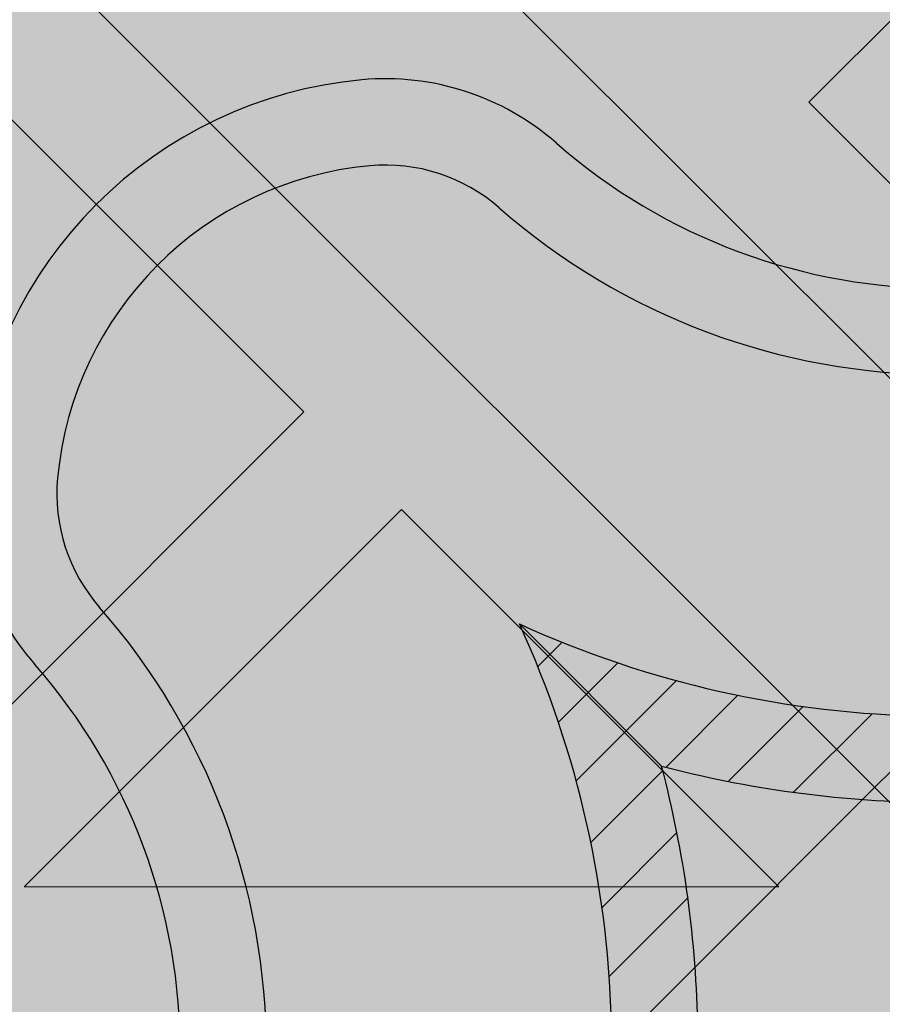
# Model space of a CAD drawing. Units: inches. Extents: x 844 to 2234, y 346 to 1084.
# Tile 17 of 93: x 1118.565 to 1120.159, y 703.242 to 705.06. Entities that reach past the tile are written whole.
import ezdxf

# ---------------------------------------------------------------- set-up
doc = ezdxf.new("R2010")
doc.units = ezdxf.units.IN
doc.header["$MEASUREMENT"] = 0
for name, color, linetype, lineweight in [('A-ANNO-DIMS', 2, 'Continuous', 18), ('furniture', 8, 'Continuous', 18), ('RA-AP-01$0$INT', 35, 'Continuous', 5)]:
    doc.layers.add(name, color=color, linetype=linetype, lineweight=lineweight)
doc.layers.add('RA-AP-01$0$FURN', color=3, linetype='Continuous')
doc.layers.add('RA-AP-01$0$WOOD', color=64, linetype='Continuous')
doc.styles.get("Standard").update_dxf_attribs({"font": 'arial.ttf'})
doc.dimstyles.get("Standard").update_dxf_attribs({"dimtxt": 6, "dimasz": 3, "dimexe": 0.18, "dimexo": 0.0625, "dimgap": 0.09, "dimtad": 0, "dimtih": 1, "dimtoh": 1, "dimdec": 1, "dimzin": 0, "dimdsep": 46, "dimlunit": 3, "dimtxsty": 'Standard', "dimblk": 'ARCHTICK', "dimcen": 0.09, "dimadec": 0, "dimazin": 0, "dimtfac": 1, "dimtdec": 1, "dimtofl": 0, "dimtmove": 0, "dimatfit": 3, "dimfxl": 1, "dimtolj": 1, "dimtzin": 0, "dimarcsym": 0})

# ---------------------------------------------------------------- blocks, each defined once
blk = doc.blocks.new('A$C18D01794')
at = {"layer": 'RA-AP-01$0$INT'}
h = blk.add_hatch(color=256, dxfattribs=at)
h.paths.add_polyline_path([(4.585917135068448, -7.856712009587804), (4.614201406330596, -7.856712009587056), (4.668846067270487, -7.802067348644738), (4.723490728212344, -7.856712009584164), (4.771774999457151, -7.856712009582887), (4.826419660396886, -7.80206734864072), (4.862780050090322, -7.838427738332541), (4.844495778842715, -7.856712009580965), (4.862780050090411, -7.856712009580482), (4.905206456960182, -7.814285602707865), (4.947632863832445, -7.856712009578238), (4.965917135079675, -7.856712009577755), (4.947632863831759, -7.838427738330656), (4.983993253523576, -7.802067348637219), (5.038637914464627, -7.856712009575829), (5.08692218571208, -7.856712009574554), (5.141566846649976, -7.802067348634224), (5.196211507589851, -7.856712009571666), (5.224495778822615, -7.856712009570916), (4.905206456953975, -7.537422687702283)])
h.paths.add_polyline_path([(4.895206456956031, -7.575706958950402), (4.895206456958921, -7.684996280828174), (4.840561796018589, -7.630351619890275)], flags=16)
h.paths.add_polyline_path([(4.915206456955638, -7.575706958949956), (4.969851117895509, -7.630351619887399), (4.915206456957609, -7.684996280827732)], flags=16)
h.paths.add_polyline_path([(4.826419660395175, -7.644493755514321), (4.881064321335613, -7.699138416452331), (4.771774999456703, -7.69913841645522)], flags=16)
h.paths.add_polyline_path([(4.983993253519558, -7.644493755510815), (5.038637914460456, -7.699138416449285), (4.929348592581548, -7.69913841645126)], flags=16)
h.paths.add_polyline_path([(4.881064321336025, -7.719138416452334), (4.826419660397532, -7.773783077393256), (4.771774999457062, -7.719138416455217)], flags=16)
h.paths.add_polyline_path([(4.929348592582019, -7.71913841645126), (5.038637914460982, -7.719138416449284), (4.983993253522945, -7.773783077389749)], flags=16)
h.paths.add_polyline_path([(4.895206456960191, -7.733280552075633), (4.895206456962115, -7.806001331460164), (4.876922185715016, -7.824285602708492), (4.840561796021581, -7.787925213016675)], flags=16)
h.paths.add_polyline_path([(4.915206456958487, -7.733280552075187), (4.969851117899527, -7.787925213013798), (4.933490728206909, -7.824285602708034), (4.9152064569598, -7.806001331461736)], flags=16)
h.paths.add_polyline_path([(4.757632863832376, -7.733280552079264), (4.812277524772842, -7.787925213017304), (4.757632863834348, -7.842569873958233)], flags=16)
h.paths.add_polyline_path([(4.737632863832376, -7.73328055207979), (4.737632863834348, -7.842569873958701), (4.682988202893906, -7.787925213020692)], flags=16)
h.paths.add_polyline_path([(5.05278005008503, -7.733280552072701), (5.052780050087917, -7.842569873951664), (4.998135389146995, -7.787925213013169)], flags=16)
h.paths.add_polyline_path([(5.072780050085024, -7.733280552072333), (5.127424711025931, -7.787925213010806), (5.072780050087916, -7.842569873951244)], flags=16)
h.paths.add_polyline_path([(4.935917135072783, -7.506712009583784), (5.255206456948811, -7.826001331459767), (5.255206456948932, -7.797717060211899), (5.200561796010279, -7.743072399273238), (5.255206456949403, -7.688427738334128), (5.25520645694961, -7.640143467086677), (5.200561796009787, -7.585498806146837), (5.236922185702417, -7.549138416454212), (5.255206456949919, -7.56742268770172), (5.255206456949998, -7.549138416454178), (5.212780050078687, -7.506712009583814), (5.25520645695036, -7.464285602712145), (5.255206456950438, -7.446001331464763), (5.236922185702424, -7.464285602712779), (5.200561796009796, -7.427925213020149), (5.255206456950753, -7.373280552079203), (5.25520645695096, -7.324996280834394), (5.200561796010322, -7.270351619893748), (5.255206456951428, -7.215706958952649), (5.255206456951547, -7.187422687705071)])
h.paths.add_polyline_path([(5.042988202883395, -7.42792521302065), (5.097632863823085, -7.373280552080975), (5.097632863822622, -7.482569873959883)], flags=16)
h.paths.add_polyline_path([(5.028846067259663, -7.442067348644384), (5.083490728198774, -7.496712009583504), (4.974201406321001, -7.496712009583035)], flags=16)
h.paths.add_polyline_path([(5.117632863823087, -7.37328055208089), (5.172277524762331, -7.42792521302015), (5.11763286382262, -7.482569873959851)], flags=16)
h.paths.add_polyline_path([(5.08349072819877, -7.516712009582191), (5.028846067259652, -7.571356670521302), (4.974201406320998, -7.516712009582638)], flags=16)
h.paths.add_polyline_path([(5.131774999446817, -7.35913841645716), (5.186419660386065, -7.413783077396415), (5.241064321325782, -7.359138416456712)], flags=17)
h.paths.add_polyline_path([(5.131774999446228, -7.496712009583703), (5.186419660386065, -7.442067348643883), (5.222780050079488, -7.478427738337313), (5.204495778832781, -7.496712009584014)], flags=16)
h.paths.add_polyline_path([(5.097632863822613, -7.530854145205813), (5.097632863823061, -7.640143467084723), (5.042988202883383, -7.585498806145032)], flags=16)
h.paths.add_polyline_path([(5.131774999446899, -7.339138416457162), (5.241064321325809, -7.339138416456712), (5.186419660386591, -7.284493755517479)], flags=17)
h.paths.add_polyline_path([(5.131774999446226, -7.516712009581999), (5.204495778830767, -7.516712009581702), (5.22278005007868, -7.534996280829206), (5.186419660386049, -7.571356670521828)], flags=16)
h.paths.add_polyline_path([(5.11763286382262, -7.530854145205852), (5.17227752476232, -7.585498806145562), (5.117632863823064, -7.64014346708481)], flags=16)
h.paths.add_polyline_path([(5.186419660386069, -7.599640941770585), (5.241064321325754, -7.654285602710281), (5.131774999446791, -7.654285602709814)], flags=16)
h.paths.add_polyline_path([(5.131774999446872, -7.674285602709813), (5.24106432132578, -7.674285602710282), (5.186419660386554, -7.728930263649504)], flags=16)
h.paths.add_polyline_path([(5.255206456951811, -7.126001331467467), (5.255206456951895, -7.106712009588038), (4.555206456956052, -7.106712009588038), (4.555206456956136, -7.12600133146746), (4.905206456953973, -7.476001331465289)])
h.paths.add_polyline_path([(4.983993253513404, -7.368930263651977), (4.92934859257295, -7.314285602713969), (5.03863791445186, -7.314285602711063)], flags=16)
h.paths.add_polyline_path([(4.969851117889988, -7.383072399276016), (4.915206456952556, -7.437717060215906), (4.915206456949648, -7.328427738338133)], flags=16)
h.paths.add_polyline_path([(4.929348592572535, -7.294285602713971), (4.983993253511019, -7.239640941773039), (5.038637914451496, -7.294285602711065)], flags=16)
h.paths.add_polyline_path([(5.052780050074912, -7.280143467087016), (4.998135389134438, -7.225498806148989), (5.052780050072919, -7.170854145208052)], flags=16)
h.paths.add_polyline_path([(5.07278005007491, -7.280143467086489), (5.072780050072918, -7.170854145207579), (5.127424711013374, -7.225498806145578)], flags=16)
h.paths.add_polyline_path([(4.89520645695295, -7.437717060216355), (4.840561796013067, -7.383072399278919), (4.895206456950961, -7.328427738338582)], flags=16)
h.paths.add_polyline_path([(4.915206456948365, -7.280143467090674), (4.915206456946434, -7.207422687704125), (4.933490728192729, -7.18913841645701), (4.969851117886972, -7.225498806149623)], flags=16)
h.paths.add_polyline_path([(4.881064321327021, -7.314285602715054), (4.82641966038902, -7.368930263655506), (4.771774999448108, -7.314285602717047)], flags=16)
h.paths.add_polyline_path([(4.895206456950073, -7.280143467091125), (4.840561796009022, -7.225498806152518), (4.876922185700835, -7.18913841645908), (4.895206456948749, -7.207422687706589)], flags=16)
h.paths.add_polyline_path([(4.983993253510392, -7.211356670525576), (4.947632863816944, -7.174996280833758), (4.965917135064043, -7.156712009585847), (5.038637914448995, -7.156712009584522)], flags=16)
h.paths.add_polyline_path([(4.881064321326543, -7.294285602715056), (4.771774999447578, -7.294285602717046), (4.826419660385607, -7.239640941776569)], flags=16)
h.paths.add_polyline_path([(4.905206456946447, -7.19913841645844), (4.862780050074785, -7.156712009587725), (4.947632863816685, -7.156712009586302)], flags=16)
h.paths.add_polyline_path([(5.14156684663679, -7.211356670521528), (5.086922185696452, -7.156712009583639), (5.196211507574223, -7.156712009581651)], flags=16)
h.paths.add_polyline_path([(4.8264196603837, -7.211356670529104), (4.771774999442643, -7.156712009590501), (4.8444957788276, -7.156712009588568), (4.862780050075511, -7.17499628083566)], flags=16)
h.paths.add_polyline_path([(4.812277524760289, -7.225498806153156), (4.757632863822258, -7.28014346709363), (4.757632863819352, -7.170854145214669)], flags=16)
h.paths.add_polyline_path([(4.73763286382226, -7.280143467093997), (4.682988202881349, -7.22549880615554), (4.737632863819352, -7.170854145215086)], flags=16)
h.paths.add_polyline_path([(4.723490728195188, -7.156712009591787), (4.668846067257299, -7.211356670532127), (4.614201406317417, -7.156712009594693)], flags=16)
h.paths.add_polyline_path([(4.597632863829262, -7.506712009583814), (4.555206456957951, -7.54913841645418), (4.555206456958029, -7.56742268770172), (4.573490728205535, -7.549138416454212), (4.609851117898167, -7.585498806146839), (4.555206456958338, -7.640143467086675), (4.555206456958546, -7.688427738334125), (4.60985111789767, -7.743072399273238), (4.555206456959015, -7.797717060211899), (4.555206456959138, -7.826001331459767), (4.874495778835167, -7.506712009583786), (4.5552064569564, -7.187422687705062), (4.555206456956523, -7.215706958952644), (4.609851117897629, -7.270351619893746), (4.555206456956988, -7.324996280834396), (4.555206456957198, -7.373280552079195), (4.609851117898153, -7.427925213020147), (4.573490728205528, -7.464285602712779), (4.555206456957507, -7.446001331464756), (4.555206456957585, -7.464285602712143)])
h.paths.add_polyline_path([(4.712780050085332, -7.482569873959882), (4.712780050084863, -7.373280552080972), (4.767424711024555, -7.42792521302065)], flags=16)
h.paths.add_polyline_path([(4.726922185709173, -7.496712009583504), (4.781566846648288, -7.442067348644384), (4.836211507586949, -7.496712009583033)], flags=16)
h.paths.add_polyline_path([(4.692780050085327, -7.482569873959851), (4.638135389145619, -7.427925213020149), (4.692780050084865, -7.373280552080892)], flags=16)
h.paths.add_polyline_path([(4.726922185709182, -7.516712009582191), (4.836211507586949, -7.51671200958264), (4.7815668466483, -7.571356670521304)], flags=16)
h.paths.add_polyline_path([(4.678637914461726, -7.496712009583706), (4.605917135075169, -7.496712009584014), (4.587632863828464, -7.478427738337311), (4.623993253521887, -7.442067348643881)], flags=16)
h.paths.add_polyline_path([(4.712780050085336, -7.530854145205816), (4.767424711024568, -7.585498806145034), (4.71278005008489, -7.640143467084724)], flags=16)
h.paths.add_polyline_path([(4.678637914461726, -7.516712009582001), (4.623993253521899, -7.571356670521829), (4.587632863829271, -7.534996280829206), (4.605917135077185, -7.5167120095817)], flags=16)
h.paths.add_polyline_path([(4.692780050085336, -7.530854145205848), (4.692780050084889, -7.64014346708481), (4.638135389145632, -7.585498806145562)], flags=16)
h.paths.add_polyline_path([(4.623993253521885, -7.413783077396415), (4.678637914461131, -7.359138416457161), (4.56934859258217, -7.359138416456712)], flags=17)
h.paths.add_polyline_path([(4.623993253521901, -7.599640941770568), (4.678637914461158, -7.654285602709814), (4.569348592582195, -7.654285602710281)], flags=16)
h.paths.add_polyline_path([(4.678637914461051, -7.339138416457162), (4.623993253521361, -7.284493755517479), (4.569348592582143, -7.339138416456712)], flags=17)
h.paths.add_polyline_path([(4.678637914461076, -7.674285602709813), (4.623993253521399, -7.728930263649504), (4.569348592582167, -7.674285602710281)], flags=16)
h = blk.add_hatch(color=256, dxfattribs=at)
h.paths.add_polyline_path([(4.905206456954232, -7.537422687702028), (4.874495778835232, -7.506712009583718), (4.555206456959138, -7.826001331459766), (4.555206456959269, -7.856712009588616), (4.585917135068449, -7.856712009587804)])
h.paths.add_polyline_path([(4.935917135072152, -7.506712009583152), (4.905206456953497, -7.537422687701806), (5.224495778822614, -7.856712009570917), (5.255206456948681, -7.856712009570104), (5.255206456948813, -7.826001331459768)])
h.paths.add_polyline_path([(5.255206456951549, -7.18742268770507), (5.255206456951813, -7.126001331467461), (4.905206456953563, -7.476001331465701), (4.935917135072559, -7.506712009584006)])
h.paths.add_polyline_path([(4.874495778835167, -7.506712009583785), (4.905206456953818, -7.476001331465132), (4.555206456956135, -7.126001331467458), (4.555206456956399, -7.187422687705064)])
h = blk.add_hatch(color=256, dxfattribs=at)
h.paths.add_polyline_path([(4.781566846647504, -7.442067348645805), (4.836211507586161, -7.496712009584463), (4.726922185708388, -7.496712009584918)])
h.paths.add_polyline_path([(4.836211507586161, -7.516712009584068), (4.781566846647504, -7.571356670522723), (4.726922185708388, -7.516712009583606)])
h.paths.add_polyline_path([(4.76742471102377, -7.585498806146453), (4.712780050084083, -7.640143467086137), (4.712780050084542, -7.530854145207227)])
h.paths.add_polyline_path([(4.692780050084544, -7.530854145207257), (4.692780050084084, -7.64014346708622), (4.638135389144834, -7.585498806146965)])
h.paths.add_polyline_path([(4.678637914460932, -7.516712009583407), (4.623993253521102, -7.571356670523233), (4.587632863827676, -7.53499628082981), (4.605917135074382, -7.516712009583104)])
h.paths.add_polyline_path([(4.573490728204743, -7.54913841645434), (4.60985111789737, -7.585498806146969), (4.555206456957541, -7.640143467086797), (4.555206456957237, -7.567422687701846)])
h.paths.add_polyline_path([(4.623993253521098, -7.599640941770699), (4.67863791446035, -7.654285602709951), (4.56934859258139, -7.654285602710407)])
h.paths.add_polyline_path([(4.678637914460275, -7.67428560270995), (4.623993253520583, -7.728930263649637), (4.56934859258136, -7.674285602710405)])
h.paths.add_polyline_path([(4.609851117896854, -7.743072399273369), (4.555206456958196, -7.797717060212026), (4.555206456957738, -7.688427738334254)])
h.paths.add_polyline_path([(4.597632863828475, -7.506712009583301), (4.555206456957283, -7.549138416454495), (4.555206456956805, -7.464285602712587)])
h.paths.add_polyline_path([(4.678637914460932, -7.496712009585113), (4.605917135076396, -7.496712009585417), (4.587632863828479, -7.478427738337913), (4.623993253521104, -7.442067348645284)])
h.paths.add_polyline_path([(4.692780050084091, -7.373280552082301), (4.692780050084548, -7.482569873961267), (4.638135389144834, -7.427925213021552)])
h.paths.add_polyline_path([(4.767424711023772, -7.427925213022072), (4.712780050084545, -7.48256987396129), (4.712780050084089, -7.373280552082384)])
h.paths.add_polyline_path([(4.67863791446036, -7.359138416457298), (4.623993253521105, -7.41378307739655), (4.569348592581399, -7.35913841645684)])
h.paths.add_polyline_path([(4.609851117897371, -7.427925213020278), (4.573490728204743, -7.464285602712907), (4.555206456957237, -7.446001331465401), (4.555206456957548, -7.373280552080448)])
h.paths.add_polyline_path([(4.623993253520596, -7.284493755517612), (4.67863791446028, -7.339138416457299), (4.569348592581367, -7.339138416456838)])
h.paths.add_polyline_path([(4.609851117896867, -7.270351619893878), (4.555206456957749, -7.324996280832994), (4.55520645695821, -7.21570695895522)])
h = blk.add_hatch(color=256, dxfattribs=at)
h.paths.add_polyline_path([(4.969851117891331, -7.630351619889621), (4.915206456952669, -7.575706958950966), (4.915206456952222, -7.684996280828739)])
h.paths.add_polyline_path([(4.895206456953064, -7.575706958950968), (4.840561796014413, -7.630351619889628), (4.895206456953533, -7.684996280828741)])
h.paths.add_polyline_path([(4.826419660390684, -7.644493755513362), (4.771774999451003, -7.699138416453052), (4.881064321329913, -7.699138416452587)])
h.paths.add_polyline_path([(4.881064321329884, -7.719138416452585), (4.771774999450921, -7.719138416453052), (4.82641966039018, -7.773783077392298)])
h.paths.add_polyline_path([(4.895206456953734, -7.733280552076196), (4.840561796013912, -7.787925213016031), (4.876922185707337, -7.824285602709455), (4.895206456954043, -7.806001331462747)])
h.paths.add_polyline_path([(4.862780050082808, -7.838427738332388), (4.826419660390178, -7.802067348639763), (4.771774999450351, -7.856712009579595), (4.844495778835303, -7.856712009579895)])
h.paths.add_polyline_path([(4.812277524766446, -7.787925213016036), (4.757632863827191, -7.733280552076788), (4.757632863826741, -7.842569873955747)])
h.paths.add_polyline_path([(4.737632863827191, -7.733280552076863), (4.682988202887508, -7.787925213016558), (4.737632863826743, -7.842569873955778)])
h.paths.add_polyline_path([(4.668846067263777, -7.802067348640287), (4.614201406325123, -7.856712009578949), (4.723490728202894, -7.856712009579402)])
h.paths.add_polyline_path([(4.905206456953846, -7.814285602708654), (4.862780050082654, -7.856712009579847), (4.947632863824561, -7.85671200958032)])
h.paths.add_polyline_path([(4.915206456952028, -7.733280552076195), (4.91520645695173, -7.806001331460731), (4.933490728199234, -7.824285602708648), (4.96985111789186, -7.787925213016022)])
h.paths.add_polyline_path([(5.038637914454841, -7.719138416453029), (4.929348592575874, -7.71913841645258), (4.983993253515593, -7.773783077392289)])
h.paths.add_polyline_path([(4.983993253515065, -7.644493755513352), (4.929348592575849, -7.699138416452582), (5.038637914454755, -7.699138416453031)])
h.paths.add_polyline_path([(5.052780050079843, -7.73328055207676), (4.998135389140595, -7.787925213016018), (5.052780050080309, -7.842569873955721)])
h.paths.add_polyline_path([(4.983993253516868, -7.802067348639752), (4.947632863824241, -7.838427738332383), (4.965917135071747, -7.856712009579888), (5.038637914456701, -7.856712009579572)])
h.paths.add_polyline_path([(5.127424711019533, -7.787925213016519), (5.072780050079843, -7.733280552076838), (5.07278005008031, -7.842569873955751)])
h.paths.add_polyline_path([(5.141566846643269, -7.802067348640248), (5.086922185704154, -7.85671200957937), (5.196211507581929, -7.856712009578901)])
for p, q in [((4.874495778835167, -7.506712009583786), (4.555206456959136, -7.826001331459769)), ((4.905206456953975, -7.537422687702283), (4.585917135071132, -7.856712009585121)), ((4.569348592582168, -7.674285602710281), (4.623993253521399, -7.728930263649504)), ((4.678637914461078, -7.674285602709813), (4.569348592582168, -7.674285602710281)), ((4.6239932535214, -7.728930263649502), (4.678637914461078, -7.674285602709813)), ((4.555206456958551, -7.68842773833413), (4.60985111789767, -7.743072399273238)), ((4.682988202893908, -7.78792521302069), (4.737632863832376, -7.733280552079792)), ((4.555206456959017, -7.797717060211899), (4.60985111789767, -7.743072399273238)), ((4.737632863834348, -7.842569873958701), (4.682988202893906, -7.787925213020692))]:
    blk.add_line(p, q, dxfattribs=at)
blk = doc.blocks.new('A$C32926AE1')
at = {"layer": 'RA-AP-01$0$WOOD'}
h = blk.add_hatch(color=256, dxfattribs=at)
h.dxf.hatch_style = 1
h.paths.add_polyline_path([(5.157430609644524, 4.573483066760929, -0.1009492694046607), (5.155401577623758, 4.593365984175333, -0.1842662638101597), (5.172249623284174, 4.638795604568598, 0.2056608120311276), (5.179560981299304, 4.661316324430096, 0.3614336704623542), (5.134352340494423, 4.706524965234944, 0.2056608120311297), (5.111831620632933, 4.699213607219793, -0.1842662638101113), (5.066402000239693, 4.682365561559342, -0.1055311479399994), (5.045656153913092, 4.68467289944697, 0.1567636581983829), (4.763886414745334, 4.684672899446966, -0.1055311479399895), (4.743140568418733, 4.68236556155934, -0.1842662638100833), (4.6977109480255, 4.69921360721979, 0.2056608120302612), (4.675190228164109, 4.706524965234949, 0.3614336704708441), (4.629981587358889, 4.66131632442871, 0.2056608120245944), (4.637292945374126, 4.638795604567974, -0.1842662638101024), (4.654140991034615, 4.59336598417475, -0.1009492694055169), (4.652111959013835, 4.573483066760181, 0.021410119221476), (4.629748025606143, 4.156712009541676, 0.0214101192214795), (4.652111959013809, 3.739940952323101, -0.1009492694059586), (4.654140991034615, 3.720058034908448, -0.1842662638100975), (4.637292945374126, 3.674628414515226, 0.2056608120245705), (4.629981587358889, 3.652107694654492, 0.3614336704708879), (4.675190228164113, 3.606899053848249, 0.2056608120302384), (4.697710948025501, 3.614210411863408, -0.1842662638100995), (4.743140568418738, 3.63105845752386, -0.1055311479402541), (4.763886414745388, 3.628751119636215, 0.1567636581983776), (5.045656153913137, 3.628751119636244, -0.1055311479397538), (5.066402000239692, 3.631058457523857, -0.1842662638101067), (5.111831620632931, 3.614210411863407, 0.2056608120310924), (5.134352340494417, 3.606899053848256, 0.3614336704624001), (5.179560981299307, 3.652107694653103, 0.2056608120311314), (5.172249623284175, 3.6746284145146, -0.1842662638101402), (5.155401577623758, 3.72005803490786, -0.1009492694051366), (5.15743060964455, 3.739940952322354, 0.0214101192215073), (5.179794543052287, 4.156712009541468, 0.0214101192215252)])
h.paths.add_polyline_path([(4.639748609479751, 4.156712009541513, 0.0213537860821624), (4.661970494867118, 3.741887061152232, -0.094075836301374), (4.664143710413708, 3.7196126951003, -0.1824818158568985), (4.644813765429836, 3.668037719127816, 0.2056608120245319), (4.639939526753007, 3.653023905887301, 0.3614336704710246), (4.676106439397173, 3.616856993242342, 0.2056608120302234), (4.691120252638095, 3.621731231919122, -0.1824818158602558), (4.742695228611606, 3.641061176902986, -0.1029891339458722), (4.766991894714349, 3.638256818950944, 0.156709409989566), (5.042550673941472, 3.638256818950105, -0.102989133958497), (5.066847340047078, 3.641061176902949, -0.1824818158594995), (5.118422316020358, 3.621731231919103, 0.2056608120311416), (5.133436129261316, 3.616856993242346, 0.3614336704621468), (5.169603041905217, 3.653023905886178, 0.2056608120310986), (5.164728803228477, 3.668037719127177, -0.1824818158565612), (5.145398858244737, 3.719612695099578, -0.0940758363009313), (5.147572073791232, 3.741887061151398, 0.0213537860822023), (5.169793959178681, 4.156712009541451, 0.0213537860822226), (5.147572073791203, 4.571536957931898, -0.0940758363005034), (5.145398858244737, 4.59381132398362, -0.1824818158565587), (5.164728803228476, 4.645386299956021, 0.2056608120311045), (5.169603041905216, 4.66040011319702, 0.3614336704621845), (5.133436129261313, 4.696567025840856, 0.2056608120310773), (5.118422316020359, 4.691692787164098, -0.182481815859508), (5.066847340047078, 4.67236284218025, -0.1029891339584606), (5.04255067394148, 4.675167200133092, 0.156709409989566), (4.766991894714357, 4.675167200132257, -0.1029891339458842), (4.742695228611611, 4.672362842180213, -0.1824818158602725), (4.691120252638095, 4.691692787164077, 0.2056608120302152), (4.676106439397174, 4.696567025840858, 0.3614336704710363), (4.639939526753005, 4.660400113195899, 0.2056608120245495), (4.644813765429837, 4.645386299955384, -0.1824818158568934), (4.664143710413708, 4.593811323982902, -0.0940758363009187), (4.661970494867149, 4.571536957931074, 0.021353786082177)], flags=16)
h.paths.add_polyline_path([(5.129794543052235, 4.432167055276933, -0.0141661062790638), (5.130152669293814, 4.156927903047693, -0.0141661062790647), (5.129794543052234, 3.881688750818433, -0.0785247771143638), (5.10979738006795, 3.755143611847103, 0.0945969212073497), (5.105408519571111, 3.717898134952927, 0.1043170707844957), (5.116074640131521, 3.670385395016088, 0.1043170707864965), (5.068561900193738, 3.681051515576561, 0.09459692119553), (5.031316423304057, 3.676662655080835, -0.1580239521427272), (4.778226145355827, 3.676662655080367, 0.0945969211986668), (4.740980668464973, 3.681051515576592, 0.1043170707882822), (4.693467928526415, 3.670385395015844, 0.1043170707867916), (4.704134049087309, 3.717898134953662, 0.0945969211972894), (4.69974518859162, 3.755143611844042, -0.0785247771163196), (4.679748025606343, 3.881688750818406, -0.0141661062790663), (4.679389899364763, 4.156927903047693, -0.0141661062790672), (4.679748025606343, 4.432167055276998, -0.0785247771163064), (4.699745188591625, 4.55871219425134, 0.094596921197333), (4.704134049087308, 4.595957671141738, 0.1043170707867205), (4.693467928526416, 4.643470411079523, 0.1043170707882628), (4.740980668464965, 4.632804290518776, 0.0945969211988114), (4.778226145355874, 4.637193151015016, -0.158023952142669), (5.031316423304015, 4.637193151014546, 0.0945969211956361), (5.068561900193736, 4.632804290518806, 0.1043170707864979), (5.11607464013152, 4.643470411079278, 0.1043170707844617), (5.105408519571112, 4.595957671142455, 0.0945969212074597), (5.109797380067959, 4.558712194248236, -0.0785247771143467)], flags=0)
h.paths.add_polyline_path([(5.119794532311105, 4.432259799204851, -0.0142000800617244), (5.120156169157484, 4.156927903047701, -0.0142000800617277), (5.119794532311105, 3.881596006890482, -0.0784894509520253), (5.100273383573699, 3.758192358677797, 0.0940138827242913), (5.095413455884425, 3.717477693979438, 0.0606271852308753), (5.099615656341024, 3.686844378806616, 0.0606271852322524), (5.068982341167493, 3.691046579263239, 0.0940138827010453), (5.028267676478798, 3.686186651576848, -0.1580706864508061), (4.781274892180912, 3.686186651576435, 0.0940138827026903), (4.740560227491556, 3.691046579263279, 0.0606271852339895), (4.709926912317155, 3.686844378806508, 0.0606271852329405), (4.714129112773991, 3.717477693980356, 0.094013882701304), (4.709269185087677, 3.758192358669163, -0.0784894509577193), (4.689748036347473, 3.881596006890469, -0.014200080061729), (4.689386399501094, 4.156927903047709, -0.0142000800617217), (4.689748036347473, 4.432259799204808, -0.078489450957724), (4.709269185087651, 4.555663447426125, 0.0940138827014585), (4.714129112773992, 4.596378112114996, 0.0606271852329731), (4.709926912317154, 4.62701142728886, 0.0606271852340196), (4.74056022749157, 4.622809226832087, 0.0940138827024997), (4.781274892180847, 4.627669154518912, -0.1580706864508359), (5.028267676478777, 4.627669154518526, 0.0940138827010946), (5.068982341167492, 4.622809226832129, 0.060627185232254), (5.099615656341024, 4.627011427288751, 0.0606271852308727), (5.095413455884425, 4.59637811211593, 0.0940138827241088), (5.100273383573675, 4.555663447417647, -0.0784894509520978)], flags=0)
h.paths.add_polyline_path([(5.06978912287499, 4.430218106756144, -0.014241683694547), (5.070173729147532, 4.156927903047672, -0.0142416836945458), (5.06978912287499, 3.883637699339223, -0.0800609523125196), (5.052662118612511, 3.773463122773442, 0.0526421978001116), (5.04590916754064, 3.740550867606997, 0.0526421977992423), (5.012996912374707, 3.73379791653534, -0.1583028414718258), (4.796545656286308, 3.73379791653451, 0.0526421978034211), (4.763633401117837, 3.740550867607021, 0.0526421978018622), (4.756880450045755, 3.773463122774558, -0.0800609523117106), (4.739753445783639, 3.883637699339268, -0.0142416836945435), (4.739368839511098, 4.156927903047671, -0.0142416836945477), (4.739753445783639, 4.430218106756155, -0.0800609523116345), (4.75688045004574, 4.540392683320762, 0.052642197801941), (4.763633401117837, 4.573304938488346, 0.0526421978035071), (4.796545656286361, 4.580057889560873, -0.1583028414717561), (5.012996912374669, 4.580057889560039, 0.0526421977993048), (5.04590916754064, 4.57330493848837, 0.0526421978002057), (5.052662118612529, 4.540392683321868, -0.080060952312477)], flags=0)
h.paths.add_polyline_path([(5.049789715110557, 4.43038092723357, -0.0143097550741839), (5.05018085590259, 4.156927903047715, -0.0143097550741854), (5.049789715110558, 3.883474878861827, -0.0800685599149176), (5.03362098255317, 3.779581877367999, 0.0306258898956367), (5.028241146483733, 3.758218888663947, 0.0306258898977031), (5.006878157778253, 3.75283905259408, -0.1583983521624096), (4.802664410878162, 3.752839052594731, 0.0306258898946014), (4.781301422174808, 3.758218888663924, 0.0306258898967912), (4.775921586105202, 3.779581877368794, -0.080068559914251), (4.759752853548071, 3.883474878861786, -0.0143097550741854), (4.759361712756037, 4.156927903047671, -0.0143097550741854), (4.759752853548071, 4.430380927233557, -0.0800685599142479), (4.775921586105193, 4.534273928726546, 0.0306258898968306), (4.781301422174808, 4.555636917431444, 0.0306258898945754), (4.802664410878143, 4.561016753500631, -0.1583983521624168), (5.006878157778244, 4.561016753501291, 0.0306258898977177), (5.028241146483733, 4.555636917431421, 0.0306258898958182), (5.03362098255321, 4.534273928727244, -0.080068559914796)], flags=0)
h.paths.add_polyline_path([(4.999766070382627, 4.428171244713864, -0.0143443147609634), (5.000198441819402, 4.156927903047689, -0.0143443147609612), (4.999766070382627, 3.885684561381556, -0.0784641635803329), (4.987356730658798, 3.799103304488872, -0.1506053783831347), (4.822185837999821, 3.79910330448882, -0.0784641635803318), (4.809776498276007, 3.885684561381509, -0.014344314760963), (4.809344126839227, 4.156927903047677, -0.0143443147609645), (4.809776498276007, 4.428171244713873, -0.0784641635803192), (4.822185837999822, 4.514752501606549, -0.1506053783831338), (4.987356730658798, 4.514752501606494, -0.078464163580285)], flags=0)
h.paths.add_polyline_path([(4.979755254238824, 4.42764379880488, -0.0143772539198268), (4.980205517789977, 4.156927903047693, -0.0143772539198275), (4.979755254238824, 3.886212007290489, -0.0689242507424422), (4.971183264704897, 3.815276770442801, -0.1296645318904179), (4.838359303953726, 3.815276770442746, -0.0689242507424186), (4.829787314419809, 3.886212007290419, -0.0143772539198292), (4.829337050868653, 4.156927903047653, -0.0143772539198325), (4.829787314419809, 4.427643798804946, -0.0689242507424211), (4.838359303953725, 4.498579035652621, -0.1296645318904187), (4.971183264704897, 4.498579035652565, -0.0689242507424401)], flags=0)
h = blk.add_hatch(color=256, dxfattribs=at)
h.dxf.hatch_style = 1
h.paths.add_polyline_path([(5.145398858244737, 4.59381132398362, -0.1824818158565616), (5.164728803228476, 4.645386299956021, 0.2056608120311045), (5.169603041905216, 4.66040011319702, 0.3614336704621845), (5.133436129261313, 4.696567025840856, 0.2056608120310773), (5.118422316020359, 4.691692787164098, -0.182481815859508), (5.066847340047078, 4.67236284218025, -0.1029891339584606), (5.04255067394148, 4.675167200133092, 0.156709409989566), (4.766991894714357, 4.675167200132257, -0.1029891339458842), (4.742695228611611, 4.672362842180213, -0.1824818158602725), (4.691120252638095, 4.691692787164077, 0.2056608120302152), (4.676106439397174, 4.696567025840858, 0.3614336704710363), (4.639939526753005, 4.660400113195899, 0.2056608120245495), (4.644813765429837, 4.645386299955384, -0.1824818158568934), (4.664143710413708, 4.593811323982902, -0.0940758363009187), (4.661970494867149, 4.571536957931074, 0.0213537860821772), (4.639748609479751, 4.156712009541507, 0.0213537860821625), (4.661970494867119, 3.741887061152226, -0.0940758363013071), (4.664143710413708, 3.719612695100309, -0.1824818158569294), (4.644813765429836, 3.668037719127816, 0.2056608120245319), (4.639939526753007, 3.653023905887301, 0.3614336704710246), (4.676106439397173, 3.616856993242342, 0.2056608120302234), (4.691120252638095, 3.621731231919122, -0.1824818158602558), (4.742695228611606, 3.641061176902986, -0.1029891339458722), (4.766991894714349, 3.638256818950944, 0.156709409989566), (5.042550673941472, 3.638256818950105, -0.102989133958497), (5.066847340047078, 3.641061176902949, -0.1824818158594995), (5.118422316020358, 3.621731231919103, 0.2056608120311416), (5.133436129261316, 3.616856993242346, 0.3614336704621468), (5.169603041905217, 3.653023905886178, 0.2056608120310986), (5.164728803228477, 3.668037719127177, -0.1824818158565612), (5.145398858244737, 3.719612695099578, -0.0940758363009313), (5.147572073791232, 3.741887061151398, 0.0213537860822023), (5.169793959178681, 4.156712009541451, 0.0213537860822226), (5.147572073791203, 4.571536957931898, -0.0940758363004996)])
h.paths.add_polyline_path([(5.109797380067958, 4.55871219424824, -0.0785247771143472), (5.129794543052234, 4.432167055276936, -0.0141661062790644), (5.130152669293814, 4.156927903047685, -0.014166106279066), (5.129794543052234, 3.881688750818401, -0.0785247771143517), (5.109797380067946, 3.755143611847092, 0.0945969212073132), (5.105408519571111, 3.717898134952929, 0.1043170707844995), (5.116074640131521, 3.670385395016088, 0.1043170707864965), (5.068561900193738, 3.681051515576561, 0.09459692119553), (5.031316423304057, 3.676662655080835, -0.1580239521427272), (4.778226145355827, 3.676662655080367, 0.0945969211986668), (4.740980668464973, 3.681051515576592, 0.1043170707882822), (4.693467928526415, 3.670385395015844, 0.1043170707867916), (4.704134049087309, 3.717898134953662, 0.0945969211972894), (4.69974518859162, 3.755143611844042, -0.0785247771163196), (4.679748025606343, 3.881688750818406, -0.0141661062790663), (4.679389899364763, 4.156927903047693, -0.0141661062790672), (4.679748025606343, 4.432167055276998, -0.0785247771163064), (4.699745188591625, 4.55871219425134, 0.094596921197333), (4.704134049087308, 4.595957671141738, 0.1043170707867205), (4.693467928526416, 4.643470411079523, 0.1043170707882628), (4.740980668464965, 4.632804290518776, 0.0945969211988114), (4.778226145355874, 4.637193151015016, -0.158023952142669), (5.031316423304015, 4.637193151014546, 0.0945969211956361), (5.068561900193736, 4.632804290518806, 0.1043170707864979), (5.11607464013152, 4.643470411079278, 0.1043170707844617), (5.105408519571112, 4.595957671142455, 0.0945969212074504)], flags=16)
h.paths.add_polyline_path([(5.100273383573655, 4.55566344741771, -0.0784894509521388), (5.119794532311105, 4.432259799204852, -0.0142000800617252), (5.120156169157484, 4.156927903047686, -0.014200080061726), (5.119794532311105, 3.881596006890502, -0.0784894509520446), (5.100273383573696, 3.758192358677786, 0.0940138827242721), (5.095413455884425, 3.717477693979436, 0.0606271852308692), (5.099615656341024, 3.686844378806616, 0.0606271852322522), (5.068982341167493, 3.691046579263239, 0.0940138827010453), (5.028267676478798, 3.686186651576848, -0.1580706864508061), (4.781274892180912, 3.686186651576435, 0.0940138827026903), (4.740560227491556, 3.691046579263279, 0.0606271852339895), (4.709926912317155, 3.686844378806508, 0.0606271852329405), (4.714129112773991, 3.717477693980356, 0.094013882701304), (4.709269185087677, 3.758192358669163, -0.0784894509577193), (4.689748036347473, 3.881596006890469, -0.014200080061729), (4.689386399501094, 4.156927903047709, -0.0142000800617217), (4.689748036347473, 4.432259799204808, -0.078489450957724), (4.709269185087651, 4.555663447426125, 0.0940138827014585), (4.714129112773992, 4.596378112114996, 0.0606271852329731), (4.709926912317154, 4.62701142728886, 0.0606271852340196), (4.74056022749157, 4.622809226832087, 0.0940138827024997), (4.781274892180847, 4.627669154518912, -0.1580706864508359), (5.028267676478777, 4.627669154518526, 0.0940138827010946), (5.068982341167492, 4.622809226832129, 0.060627185232254), (5.099615656341024, 4.627011427288751, 0.0606271852308727), (5.095413455884425, 4.59637811211593, 0.094013882723957)], flags=0)
h.paths.add_polyline_path([(5.04590916754064, 4.57330493848837, 0.0526421978002057), (5.052662118612529, 4.540392683321868, -0.0800609523124783), (5.06978912287499, 4.430218106756142, -0.0142416836945469), (5.070173729147532, 4.156927903047672, -0.0142416836945458), (5.06978912287499, 3.883637699339223, -0.0800609523125196), (5.052662118612511, 3.773463122773442, 0.0526421978001116), (5.04590916754064, 3.740550867606997, 0.0526421977992423), (5.012996912374707, 3.73379791653534, -0.1583028414718258), (4.796545656286308, 3.73379791653451, 0.0526421978034211), (4.763633401117837, 3.740550867607021, 0.0526421978018622), (4.756880450045755, 3.773463122774558, -0.0800609523117106), (4.739753445783639, 3.883637699339268, -0.0142416836945435), (4.739368839511098, 4.156927903047671, -0.0142416836945477), (4.739753445783639, 4.430218106756155, -0.0800609523116345), (4.75688045004574, 4.540392683320762, 0.052642197801941), (4.763633401117837, 4.573304938488346, 0.0526421978035071), (4.796545656286361, 4.580057889560873, -0.1583028414717561), (5.012996912374669, 4.580057889560039, 0.0526421977993048)], flags=0)
h.paths.add_polyline_path([(5.028241146483733, 4.555636917431422, 0.0306258898956949), (5.033620982553182, 4.534273928727329, -0.0800685599148649), (5.049789715110557, 4.430380927233569, -0.0143097550741839), (5.05018085590259, 4.156927903047715, -0.0143097550741854), (5.049789715110558, 3.883474878861827, -0.0800685599149176), (5.03362098255317, 3.779581877367999, 0.0306258898956367), (5.028241146483733, 3.758218888663947, 0.0306258898977031), (5.006878157778253, 3.75283905259408, -0.1583983521624096), (4.802664410878162, 3.752839052594731, 0.0306258898946014), (4.781301422174808, 3.758218888663924, 0.0306258898967912), (4.775921586105202, 3.779581877368794, -0.080068559914251), (4.759752853548071, 3.883474878861786, -0.0143097550741854), (4.759361712756037, 4.156927903047671, -0.0143097550741854), (4.759752853548071, 4.430380927233557, -0.0800685599142479), (4.775921586105193, 4.534273928726546, 0.0306258898968306), (4.781301422174808, 4.555636917431444, 0.0306258898945754), (4.802664410878143, 4.561016753500631, -0.1583983521624168), (5.006878157778244, 4.561016753501291, 0.0306258898977174)], flags=0)
h.paths.add_polyline_path([(4.987356730658798, 4.514752501606494, -0.0784641635803018), (4.999766070382627, 4.428171244713845, -0.0143443147609637), (5.000198441819402, 4.156927903047665, -0.0143443147609622), (4.999766070382628, 3.885684561381514, -0.0784641635802952), (4.987356730658797, 3.799103304488872, -0.1506053783831338), (4.822185837999821, 3.799103304488819, -0.0784641635803342), (4.809776498276007, 3.885684561381512, -0.0143443147609628), (4.809344126839227, 4.156927903047676, -0.0143443147609646), (4.809776498276007, 4.428171244713873, -0.0784641635803192), (4.822185837999822, 4.514752501606549, -0.1506053783831338)], flags=0)
h.paths.add_polyline_path([(4.971183264704897, 4.498579035652566, -0.0689242507424384), (4.979755254238824, 4.427643798804883, -0.0143772539198276), (4.980205517789977, 4.15692790304768, -0.0143772539198258), (4.979755254238823, 3.88621200729051, -0.0689242507424628), (4.971183264704897, 3.815276770442801, -0.129664531890417), (4.838359303953726, 3.815276770442746, -0.0689242507424186), (4.829787314419809, 3.886212007290419, -0.0143772539198292), (4.829337050868653, 4.156927903047653, -0.0143772539198325), (4.829787314419809, 4.427643798804946, -0.0689242507424211), (4.838359303953725, 4.498579035652621, -0.1296645318904187)], flags=0)
h = blk.add_hatch(dxfattribs=at)
h.set_pattern_fill('ANSI31', color=256, scale=0.05, style=0)
h.set_pattern_definition([(45, (0, 0), (-0.0044194173824159, 0.0044194173824159), [])])
h.paths.add_polyline_path([(5.130152669293814, 4.156927903047704, 0.0141661062790657), (5.129794543052234, 4.432167055276982, 0.0777827904001433), (5.110168979996553, 4.557559993161921, -0.0976515123401879), (5.105408519571111, 4.595957671142454, -0.1043170707844687), (5.116074640131522, 4.64347041107928), (5.099615656341024, 4.627011427288751, 0.0606271852308727), (5.095413455884425, 4.59637811211593, 0.0940138827241088), (5.100273383573675, 4.555663447417647, -0.0784894509520972), (5.119794532311105, 4.432259799204852, -0.0142000800617252), (5.120156169157484, 4.156927903047686, -0.014200080061726), (5.119794532311105, 3.881596006890502, -0.0784894509520446), (5.100273383573696, 3.758192358677786, 0.0940138827242721), (5.095413455884425, 3.717477693979436, 0.0606271852308692), (5.099615656341024, 3.686844378806616), (5.116074640131519, 3.67038539501609, -0.1043170707844594), (5.105408519571112, 3.717898134952912, -0.0976515123401594), (5.11016897999655, 3.756295812933435, 0.0777827904001654), (5.129794543052234, 3.881688750818409, 0.0141661062790665)])
h.paths.add_polyline_path([(5.030164222210597, 3.676291055149937, -0.0976515123472002), (5.068561900193739, 3.681051515576561, -0.1043170707864927), (5.116074640131521, 3.670385395016088), (5.099615656341024, 3.686844378806616, 0.0606271852322522), (5.068982341167493, 3.691046579263239, 0.0940138827010453), (5.028267676478798, 3.686186651576848, -0.1580706864508061), (4.781274892180912, 3.686186651576435, 0.0940138827026903), (4.740560227491556, 3.691046579263279, 0.0606271852339913), (4.709926912317154, 3.686844378806508), (4.693467928526416, 3.670385395015845, -0.1043170707882796), (4.740980668464973, 3.681051515576592, -0.0976515123427246), (4.779378346446416, 3.676291055150394, 0.156512506893803)])
h.paths.add_polyline_path([(4.689748036347473, 3.881596006890472, -0.014200080061729), (4.689386399501094, 4.156927903047712, -0.0142000800617195), (4.689748036347473, 4.432259799204768, -0.078489450957742), (4.709269185087648, 4.555663447426114, 0.0940138827014821), (4.714129112773992, 4.596378112114995, 0.0606271852329748), (4.709926912317154, 4.62701142728886), (4.693467928526414, 4.643470411079524, -0.1043170707867939), (4.704134049087309, 4.595957671141706, -0.09765151234893), (4.699373588660725, 4.557559993157876, 0.0777827903975372), (4.679748025606343, 4.432167055276987, 0.0141661062790675), (4.679389899364763, 4.156927903047675, 0.0141661062790641), (4.679748025606343, 3.88168875081843, 0.0777827903975637), (4.699373588660724, 3.756295812937497, -0.0976515123490278), (4.704134049087308, 3.717898134953629, -0.1043170707867196), (4.693467928526416, 3.670385395015845), (4.709926912317155, 3.686844378806508, 0.0606271852329413), (4.714129112773991, 3.717477693980357, 0.0940138827013084), (4.709269185087676, 3.758192358669166, -0.0784894509577192)])
h.paths.add_polyline_path([(4.779378346446434, 4.63756475094498, -0.0976515123427943), (4.740980668464964, 4.632804290518776, -0.1043170707882609), (4.693467928526416, 4.643470411079523), (4.709926912317154, 4.62701142728886, 0.0606271852340196), (4.74056022749157, 4.622809226832087, 0.0940138827024997), (4.781274892180847, 4.627669154518912, -0.1580706864508359), (5.028267676478777, 4.627669154518526, 0.0940138827010946), (5.068982341167492, 4.622809226832129, 0.060627185232254), (5.099615656341024, 4.627011427288751), (5.116074640131521, 4.643470411079279, -0.1043170707865022), (5.068561900193735, 4.632804290518806, -0.0976515123475899), (5.030164222210446, 4.637564750945479, 0.1565125068936924)])
h = blk.add_hatch(dxfattribs=at)
h.set_pattern_fill('ANSI32', color=256, scale=0.2, style=0)
h.set_pattern_definition([(45, (0, 0), (-0.0530330085889911, 0.0530330085889911), []), (45, (0.035355339, 0), (-0.0530330085889911, 0.0530330085889911), [])])
h.paths.add_polyline_path([(5.119794532311105, 4.432259799204823, 0.0777015974868765), (5.10065834347252, 4.554469821747928, -0.0968902511992216), (5.095413455884425, 4.596378112115931, -0.060627185230871), (5.099615656341024, 4.627011427288751, -0.060627185232254), (5.068982341167492, 4.622809226832129, -0.0968902512198245), (5.027074050790956, 4.628054114423209, 0.1564657949319105), (4.782468517866163, 4.628054114422785, -0.0968902512152247), (4.740560227491555, 4.622809226832088, -0.0606271852339878), (4.709926912317155, 4.627011427288859, -0.0606271852329413), (4.714129112773991, 4.596378112115011, -0.0968902512205338), (4.708884225182929, 4.554469821738175, 0.0777015974804443), (4.689748036347473, 4.43225979920482, 0.0142000800617215), (4.689386399501094, 4.156927903047726, 0.0142000800617273), (4.689748036347473, 3.88159600689052, 0.077701597480541), (4.708884225182985, 3.759385984357019, -0.096890251220082), (4.714129112773992, 3.717477693980371, -0.0606271852329731), (4.709926912317154, 3.686844378806507, -0.060627185233988), (4.740560227491554, 3.691046579263279, -0.0968902512152569), (4.782468517866175, 3.685801691672578, 0.1564657949319236), (5.027074050790988, 3.685801691672169, -0.0968902512197451), (5.068982341167491, 3.691046579263239, -0.0606271852322557), (5.099615656341024, 3.686844378806616, -0.0606271852308727), (5.095413455884425, 3.717477693979438, -0.0968902511991229), (5.100658343472507, 3.7593859843474, 0.0777015974868745), (5.119794532311105, 3.8815960068905, 0.014200080061726), (5.120156169157484, 4.156927903047685, 0.0142000800617238)])
h.paths.add_polyline_path([(5.070173729147531, 4.156927903047684, -0.0142416836945481), (5.06978912287499, 3.883637699339191, -0.0800609523125107), (5.052662118612505, 3.773463122773424, 0.0526421978000811), (5.04590916754064, 3.740550867606997, 0.0526421977993214), (5.012996912374658, 3.733797916535325, -0.1583028414717916), (4.796545656286304, 3.733797916534512, 0.0526421978034138), (4.763633401117837, 3.740550867607021, 0.0526421978018622), (4.756880450045755, 3.773463122774558, -0.0800609523117106), (4.739753445783639, 3.883637699339268, -0.0142416836945435), (4.739368839511098, 4.156927903047671, -0.0142416836945477), (4.739753445783639, 4.430218106756155, -0.0800609523116345), (4.75688045004574, 4.540392683320762, 0.052642197801941), (4.763633401117837, 4.573304938488346, 0.0526421978035071), (4.796545656286361, 4.580057889560873, -0.1583028414717561), (5.012996912374669, 4.580057889560039, 0.0526421977993048), (5.04590916754064, 4.57330493848837, 0.0526421978002057), (5.052662118612529, 4.540392683321868, -0.0800609523124783), (5.06978912287499, 4.430218106756142, -0.0142416836945463)], flags=16)
h.paths.add_polyline_path([(5.050180855902591, 4.156927903047686, -0.0143097550741856), (5.049789715110558, 3.883474878861795, -0.0800685599148126), (5.033620982553202, 3.7795818773681, 0.0306258898957837), (5.028241146483733, 3.758218888663947, 0.0306258898977031), (5.006878157778253, 3.75283905259408, -0.1583983521624096), (4.802664410878162, 3.752839052594731, 0.0306258898946014), (4.781301422174808, 3.758218888663924, 0.0306258898967912), (4.775921586105202, 3.779581877368794, -0.080068559914251), (4.759752853548071, 3.883474878861786, -0.0143097550741854), (4.759361712756037, 4.156927903047671, -0.0143097550741854), (4.759752853548071, 4.430380927233557, -0.0800685599142479), (4.775921586105193, 4.534273928726546, 0.0306258898968306), (4.781301422174808, 4.555636917431444, 0.0306258898945754), (4.802664410878143, 4.561016753500631, -0.1583983521624168), (5.006878157778244, 4.561016753501291, 0.0306258898977177), (5.028241146483733, 4.555636917431421, 0.0306258898958182), (5.03362098255321, 4.534273928727244, -0.0800685599147973), (5.049789715110557, 4.430380927233568, -0.0143097550741854)], flags=0)
h.paths.add_polyline_path([(5.000198441819402, 4.15692790304769, -0.0143443147609622), (4.999766070382627, 3.885684561381539, -0.0784641635803169), (4.987356730658798, 3.799103304488873, -0.1506053783831347), (4.822185837999821, 3.79910330448882, -0.0784641635803318), (4.809776498276007, 3.885684561381509, -0.014344314760963), (4.809344126839227, 4.156927903047677, -0.0143443147609645), (4.809776498276007, 4.428171244713873, -0.0784641635803192), (4.822185837999822, 4.514752501606549, -0.1506053783831338), (4.987356730658798, 4.514752501606494, -0.0784641635803018), (4.999766070382627, 4.428171244713845, -0.0143443147609624)], flags=0)
h.paths.add_polyline_path([(4.980205517789976, 4.156927903047707, -0.0143772539198295), (4.979755254238824, 3.886212007290466, -0.06892425074242), (4.971183264704897, 3.815276770442801, -0.129664531890417), (4.838359303953726, 3.815276770442746, -0.0689242507424186), (4.829787314419809, 3.886212007290419, -0.0143772539198292), (4.829337050868653, 4.156927903047653, -0.0143772539198325), (4.829787314419809, 4.427643798804946, -0.0689242507424211), (4.838359303953725, 4.498579035652621, -0.1296645318904187), (4.971183264704897, 4.498579035652565, -0.0689242507424418), (4.979755254238824, 4.427643798804878, -0.0143772539198259)], flags=0)
blk.add_line((4.709926912317154, 4.62701142728886), (4.693467928526416, 4.643470411079523), dxfattribs=at)
blk.add_line((4.709926912317154, 4.62701142728886), (4.693467928526416, 4.643470411079523), dxfattribs=at)
for centre, radius, start, end in [((4.679771284329349, 4.656735268264593), 0.0499999999998897, 95.25687599443106, 174.7431240064049), ((4.67793886186326, 4.676651147052671), 0.0299999999999992, 48.77105092035662, 95.25687599427984), ((4.742507915094499, 4.750332633143934), 0.0679700159630274, 228.7710509203537, 270.5333070513671), ((4.679771284329334, 4.656735268264609), 0.0399999999998732, 95.25687599445018, 174.7431240064249), ((4.67793886186326, 4.676651147052671), 0.0199999999999984, 48.77105092035742, 95.25687599428184), ((4.742507915094546, 4.750332633143919), 0.0779700159630467, 228.7710509203206, 270.1376463011373), ((4.659855405541232, 4.658567690730234), 0.0300000000000005, 174.7431240062535, 221.2289490796905), ((4.65985540554127, 4.658567690730245), 0.0200000000000369, 174.7431240062188, 221.2289490796444), ((4.586173919450017, 4.593998637498934), 0.077970015963029, 359.8623536996133, 41.22894907969008), ((4.586173919450015, 4.5944304245111), 0.1179700159630316, 0.7417751874182703, 24.56332695026347), ((4.742507915094493, 4.750764420156106), 0.1179700159630538, 245.436673049926, 269.258224813113), ((4.586173919450019, 4.593998637498935), 0.0679700159630267, 359.4666929486785, 41.22894907969187), ((4.586173919450018, 4.594430424511101), 0.1279700159630281, 0.8720682535796656, 14.74980897308237), ((4.742507915094622, 4.750764420156106), 0.1279700159630606, 255.250191027056, 269.1279317467988)]:
    blk.add_arc(centre, radius, start, end, dxfattribs=at)
blk = doc.blocks.new('A$C5D2F253E')
at = {"layer": 'RA-AP-01$0$FURN', "xscale": -0.7999999999883585, "yscale": 0.7999999999883585, "zscale": 0.8, "rotation": 90}
blk.add_blockref('A$C18D01794', (-5.687757199772477, 4.75791982714071), dxfattribs=at)
at = {"layer": 'RA-AP-01$0$WOOD', "rotation": 270}
blk.add_blockref('A$C32926AE1', (-4.161339601644158, 5.73852594588169), dxfattribs=at)
blk = doc.blocks.new('_ArchTick')
at = {"color": 0, "linetype": 'ByBlock', "const_width": 0.15}
blk.add_lwpolyline([(-0.5, -0.5), (0.5, 0.5)], dxfattribs=at)
blk = doc.blocks.new('*D144')
at = {"layer": 'A-ANNO-DIMS', "color": 0, "lineweight": -2, "transparency": 16777216}
for p, q in [((1096.615948, 439.3732739999999), (1096.615948, 1074.743301)), ((1143.115948, 492.373274), (1143.115948, 1074.743301)), ((1096.615948, 1074.563301), (1102.481950728513, 1074.563301)), ((1143.115948, 1074.563301), (1137.249945271487, 1074.563301))]:
    blk.add_line(p, q, dxfattribs=at)
at = {"layer": 'Defpoints', "color": 0, "transparency": 16777216}
for p in [(1143.115948, 1074.563301), (1143.115948, 492.3107739999999), (1096.615948, 439.3107739999999)]:
    blk.add_point(p, dxfattribs=at)
at = {"layer": 'A-ANNO-DIMS', "color": 0, "lineweight": -2, "transparency": 16777216, "xscale": 3, "yscale": 3, "zscale": 3, "rotation": 180}
blk.add_blockref('_ArchTick', (1096.615948, 1074.563301), dxfattribs=at)
at = {"layer": 'A-ANNO-DIMS', "color": 0, "lineweight": -2, "transparency": 16777216, "xscale": 3, "yscale": 3, "zscale": 3}
blk.add_blockref('_ArchTick', (1143.115948, 1074.563301), dxfattribs=at)
at = {"layer": 'A-ANNO-DIMS', "color": 0, "transparency": 16777216, "insert": (1119.865948, 1074.563301), "char_height": 6, "attachment_point": 5}
blk.add_mtext('\\A1;3\'-10 1/2"', dxfattribs=at)

msp = doc.modelspace()

# ---------------------------------------------------------------- block references
at = {"layer": 'furniture', "xscale": 15.94108302203742, "yscale": 15.94108302203742, "zscale": 15.94108302203742, "rotation": 90}
msp.add_blockref('A$C5D2F253E', (1136.147844094663, 696.2584716700112), dxfattribs=at)

# ---------------------------------------------------------------- dimensions: what is measured, and where the dimension line sits
at = {"layer": 'A-ANNO-DIMS'}
dim = msp.add_linear_dim(base=(1143.115948, 1074.563301), p1=(1096.615948, 439.3107739999999), p2=(1143.115948, 492.3107739999999), dimstyle='Standard', override={"dimdec": 1, "dimlfac": 1, "dimrnd": 0, "dimzin": 1, "dimdsep": 46, "dimlunit": 4, "dimfrac": 2}, dxfattribs=at)
dim.commit()
dim.dimension.update_dxf_attribs({"geometry": '*D144', "text_midpoint": (1119.865948, 1074.563301)})

doc.saveas('drawing.dxf')
